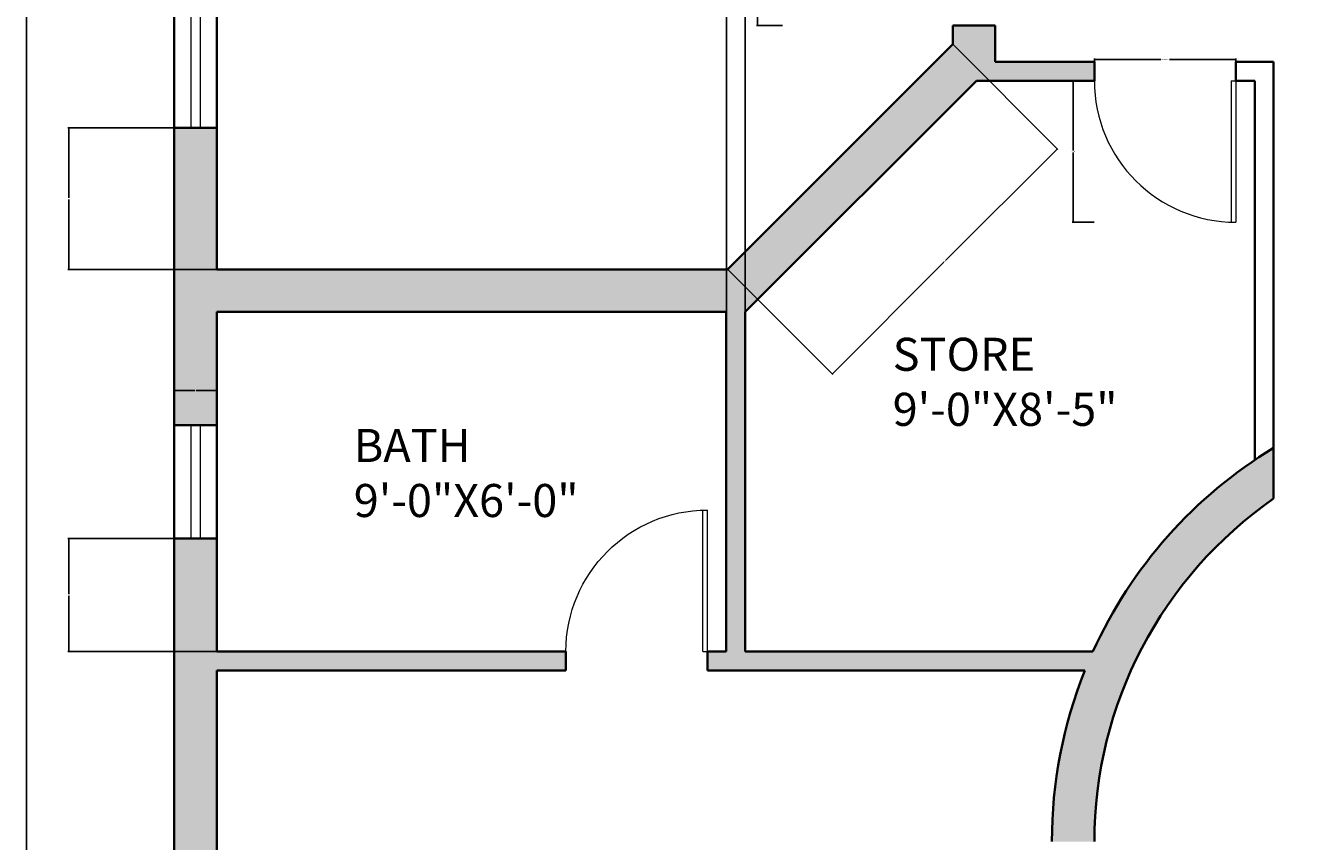
# Model space of a CAD drawing. Units: inches. Extents: x 1919 to 2461, y 2470 to 3159.
# Tile 2 of 6: x 1919 to 2188, y 2630 to 2803. Entities that reach past the tile are written whole.
import ezdxf

# ---------------------------------------------------------------- set-up
doc = ezdxf.new("R2010")
doc.units = ezdxf.units.IN
for name, color, linetype, lineweight in [('A-ANNO-DIMS', 2, 'Continuous', 18), ('A-AREA-IDEN', 7, 'Continuous', 18), ('A-DOOR', 3, 'Continuous', 18), ('A-GLAZ', 4, 'Continuous', 18), ('A-WALL', 7, 'Continuous', 35), ('A-WALL-PATT', 252, 'Continuous', 13)]:
    doc.layers.add(name, color=color, linetype=linetype, lineweight=lineweight)
doc.styles.get("Standard").update_dxf_attribs({"font": 'arial.ttf'})
doc.dimstyles.get("Standard").update_dxf_attribs({"dimtxt": 0.18, "dimasz": 0.18, "dimexe": 0.18, "dimexo": 0.0625, "dimgap": 0.09, "dimtad": 0, "dimtih": 1, "dimtoh": 1, "dimdec": 4, "dimzin": 0, "dimdsep": 46, "dimtxsty": 'Standard', "dimcen": 0.09, "dimadec": 0, "dimazin": 0, "dimtfac": 1, "dimtdec": 4, "dimtofl": 0, "dimtmove": 0, "dimatfit": 3, "dimfxl": 1, "dimtolj": 1, "dimtzin": 0, "dimarcsym": 0})

# ---------------------------------------------------------------- blocks, each defined once
blk = doc.blocks.new('DOOR-SGL-30IN')
for p, q in [((0, 0), (0, 30)), ((1, 0), (1, 29.98)), ((1, 0), (0, 0))]:
    blk.add_line(p, q)
blk.add_arc((0, 0), 30, 0, 90)
blk = doc.blocks.new('WIN-GLAZ-120IN')
for p, q in [((120, 0), (0, 0)), ((120, -2), (0, -2))]:
    blk.add_line(p, q)
blk = doc.blocks.new('WIN-GLAZ-24IN')
for p, q in [((-2, 24), (-2, 0)), ((0, 24), (0, 0))]:
    blk.add_line(p, q)
blk = doc.blocks.new('*D14')
at = {"layer": 'A-ANNO-DIMS', "color": 0, "lineweight": -2, "transparency": 16777216}
for p, q in [((2079.25, 2839.4), (2073.74, 2839.4)), ((2073.92, 2839.22), (2073.92, 2821.58)), ((2073.92, 2803.58), (2073.92, 2821.22)), ((2079.25, 2803.4), (2073.74, 2803.4))]:
    blk.add_line(p, q, dxfattribs=at)
at = {"layer": 'A-ANNO-DIMS', "color": 0, "transparency": 16777216}
for points in [[(2073.89, 2839.22), (2073.95, 2839.22), (2073.92, 2839.4)], [(2073.89, 2803.58), (2073.95, 2803.58), (2073.92, 2803.4)]]:
    blk.add_solid(points, dxfattribs=at)
at = {"layer": 'Defpoints', "color": 0, "transparency": 16777216}
for p in [(2073.92, 2839.4), (2079.32, 2839.4), (2079.32, 2803.4)]:
    blk.add_point(p, dxfattribs=at)
at = {"layer": 'A-ANNO-DIMS', "color": 0, "transparency": 16777216, "insert": (2073.92, 2821.4), "char_height": 0.18, "attachment_point": 5}
blk.add_mtext('\\A1;36 TYP.', dxfattribs=at)
blk = doc.blocks.new('*D15')
at = {"layer": 'A-ANNO-DIMS', "color": 0, "lineweight": -2, "transparency": 16777216}
for p, q in [((2145.32, 2791.73), (2145.32, 2796.35)), ((2145.5, 2796.17), (2159.38, 2796.17)), ((2175.14, 2796.17), (2161.25, 2796.17)), ((2175.32, 2791.73), (2175.32, 2796.35))]:
    blk.add_line(p, q, dxfattribs=at)
at = {"layer": 'A-ANNO-DIMS', "color": 0, "transparency": 16777216}
for points in [[(2145.5, 2796.2), (2145.5, 2796.14), (2145.32, 2796.17)], [(2175.14, 2796.2), (2175.14, 2796.14), (2175.32, 2796.17)]]:
    blk.add_solid(points, dxfattribs=at)
at = {"layer": 'Defpoints', "color": 0, "transparency": 16777216}
for p in [(2145.32, 2796.17), (2145.32, 2791.67), (2175.32, 2791.67)]:
    blk.add_point(p, dxfattribs=at)
at = {"layer": 'A-ANNO-DIMS', "color": 0, "transparency": 16777216, "insert": (2160.32, 2796.17), "char_height": 0.18, "attachment_point": 5}
blk.add_mtext('\\A1;DOOR 30 TYP.', dxfattribs=at)
blk = doc.blocks.new('*D16')
at = {"layer": 'A-ANNO-DIMS', "color": 0, "lineweight": -2, "transparency": 16777216}
for p, q in [((2145.25, 2791.67), (2140.64, 2791.67)), ((2140.82, 2791.49), (2140.82, 2776.85)), ((2140.82, 2761.85), (2140.82, 2776.49)), ((2145.25, 2761.67), (2140.64, 2761.67))]:
    blk.add_line(p, q, dxfattribs=at)
at = {"layer": 'A-ANNO-DIMS', "color": 0, "transparency": 16777216}
for points in [[(2140.79, 2791.49), (2140.85, 2791.49), (2140.82, 2791.67)], [(2140.79, 2761.85), (2140.85, 2761.85), (2140.82, 2761.67)]]:
    blk.add_solid(points, dxfattribs=at)
at = {"layer": 'Defpoints', "color": 0, "transparency": 16777216}
for p in [(2145.32, 2791.67), (2140.82, 2761.67), (2145.32, 2761.67)]:
    blk.add_point(p, dxfattribs=at)
at = {"layer": 'A-ANNO-DIMS', "color": 0, "transparency": 16777216, "insert": (2140.82, 2776.67), "char_height": 0.18, "attachment_point": 5}
blk.add_mtext('\\A1;30 TYP.', dxfattribs=at)
blk = doc.blocks.new('*D24')
at = {"layer": 'A-ANNO-DIMS', "color": 0, "lineweight": -2, "transparency": 16777216}
for p, q in [((2004.25, 3127.67), (1918.78, 3127.67)), ((1918.96, 3127.49), (1918.96, 2814.85)), ((1918.96, 2501.85), (1918.96, 2814.49)), ((1950.25, 2501.67), (1918.78, 2501.67))]:
    blk.add_line(p, q, dxfattribs=at)
at = {"layer": 'A-ANNO-DIMS', "color": 0, "transparency": 16777216}
for points in [[(1918.93, 3127.49), (1918.99, 3127.49), (1918.96, 3127.67)], [(1918.93, 2501.85), (1918.99, 2501.85), (1918.96, 2501.67)]]:
    blk.add_solid(points, dxfattribs=at)
at = {"layer": 'Defpoints', "color": 0, "transparency": 16777216}
for p in [(1918.96, 3127.67), (2004.32, 3127.67), (1950.32, 2501.67)]:
    blk.add_point(p, dxfattribs=at)
at = {"layer": 'A-ANNO-DIMS', "color": 0, "transparency": 16777216, "insert": (1918.96, 2814.67), "char_height": 0.18, "attachment_point": 5}
blk.add_mtext('\\A1;626', dxfattribs=at)
blk = doc.blocks.new('*D30')
at = {"layer": 'A-ANNO-DIMS', "color": 0, "lineweight": -2, "transparency": 16777216}
for p, q in [((1959.25, 2781.67), (1927.78, 2781.67)), ((1927.96, 2781.49), (1927.96, 2766.85)), ((1927.96, 2751.85), (1927.96, 2766.49)), ((1959.25, 2751.67), (1927.78, 2751.67))]:
    blk.add_line(p, q, dxfattribs=at)
at = {"layer": 'A-ANNO-DIMS', "color": 0, "transparency": 16777216}
for points in [[(1927.93, 2781.49), (1927.99, 2781.49), (1927.96, 2781.67)], [(1927.93, 2751.85), (1927.99, 2751.85), (1927.96, 2751.67)]]:
    blk.add_solid(points, dxfattribs=at)
at = {"layer": 'Defpoints', "color": 0, "transparency": 16777216}
for p in [(1927.96, 2781.67), (1959.32, 2781.67), (1959.32, 2751.67)]:
    blk.add_point(p, dxfattribs=at)
at = {"layer": 'A-ANNO-DIMS', "color": 0, "transparency": 16777216, "insert": (1927.96, 2766.67), "char_height": 0.18, "attachment_point": 5}
blk.add_mtext('\\A1;30', dxfattribs=at)
blk = doc.blocks.new('*D31')
at = {"layer": 'A-ANNO-DIMS', "color": 0, "lineweight": -2, "transparency": 16777216}
for p, q in [((1959.25, 2694.67), (1927.78, 2694.67)), ((1927.96, 2694.49), (1927.96, 2682.85)), ((1927.96, 2670.85), (1927.96, 2682.49)), ((1959.25, 2670.67), (1927.78, 2670.67))]:
    blk.add_line(p, q, dxfattribs=at)
at = {"layer": 'A-ANNO-DIMS', "color": 0, "transparency": 16777216}
for points in [[(1927.93, 2694.49), (1927.99, 2694.49), (1927.96, 2694.67)], [(1927.93, 2670.85), (1927.99, 2670.85), (1927.96, 2670.67)]]:
    blk.add_solid(points, dxfattribs=at)
at = {"layer": 'Defpoints', "color": 0, "transparency": 16777216}
for p in [(1927.96, 2694.67), (1959.32, 2694.67), (1959.32, 2670.67)]:
    blk.add_point(p, dxfattribs=at)
at = {"layer": 'A-ANNO-DIMS', "color": 0, "transparency": 16777216, "insert": (1927.96, 2682.67), "char_height": 0.18, "attachment_point": 5}
blk.add_mtext('\\A1;24', dxfattribs=at)
blk = doc.blocks.new('*D39')
at = {"layer": 'A-ANNO-DIMS', "color": 0, "lineweight": -2, "transparency": 16777216}
for p, q in [((2067.32, 2670.73), (2067.32, 3159.21)), ((2067.5, 3159.03), (2069.16, 3159.03)), ((2071.14, 3159.03), (2069.47, 3159.03)), ((2071.32, 2670.73), (2071.32, 3159.21))]:
    blk.add_line(p, q, dxfattribs=at)
at = {"layer": 'A-ANNO-DIMS', "color": 0, "transparency": 16777216}
for points in [[(2067.5, 3159.06), (2067.5, 3159), (2067.32, 3159.03)], [(2071.14, 3159.06), (2071.14, 3159), (2071.32, 3159.03)]]:
    blk.add_solid(points, dxfattribs=at)
at = {"layer": 'Defpoints', "color": 0, "transparency": 16777216}
for p in [(2071.32, 3159.03), (2067.32, 2670.67), (2071.32, 2670.67)]:
    blk.add_point(p, dxfattribs=at)
at = {"layer": 'A-ANNO-DIMS', "color": 0, "transparency": 16777216, "insert": (2069.32, 3159.03), "char_height": 0.18, "attachment_point": 5}
blk.add_mtext('\\A1;4', dxfattribs=at)
blk = doc.blocks.new('*D40')
at = {"layer": 'A-ANNO-DIMS', "color": 0, "lineweight": -2, "transparency": 16777216}
for p, q in [((1950.32, 2694.73), (1950.32, 2726.21)), ((1950.5, 2726.03), (1954.67, 2726.03)), ((1959.14, 2726.03), (1954.96, 2726.03)), ((1959.32, 2694.73), (1959.32, 2726.21))]:
    blk.add_line(p, q, dxfattribs=at)
at = {"layer": 'A-ANNO-DIMS', "color": 0, "transparency": 16777216}
for points in [[(1950.5, 2726.06), (1950.5, 2726), (1950.32, 2726.03)], [(1959.14, 2726.06), (1959.14, 2726), (1959.32, 2726.03)]]:
    blk.add_solid(points, dxfattribs=at)
at = {"layer": 'Defpoints', "color": 0, "transparency": 16777216}
for p in [(1959.32, 2726.03), (1950.32, 2694.67), (1959.32, 2694.67)]:
    blk.add_point(p, dxfattribs=at)
at = {"layer": 'A-ANNO-DIMS', "color": 0, "transparency": 16777216, "insert": (1954.82, 2726.03), "char_height": 0.18, "attachment_point": 5}
blk.add_mtext('\\A1;9', dxfattribs=at)
blk = doc.blocks.new('*D44')
at = {"layer": 'A-ANNO-DIMS', "color": 0, "lineweight": -2, "transparency": 16777216}
for p, q in [((2115.36, 2799.36), (2137.61, 2777.1)), ((2137.36, 2777.1), (2113.8, 2753.55)), ((2089.89, 2729.63), (2113.44, 2753.18)), ((2067.63, 2751.63), (2089.89, 2729.37))]:
    blk.add_line(p, q, dxfattribs=at)
at = {"layer": 'A-ANNO-DIMS', "color": 0, "transparency": 16777216}
for points in [[(2137.34, 2777.12), (2137.38, 2777.08), (2137.49, 2777.23)], [(2089.86, 2729.65), (2089.91, 2729.61), (2089.76, 2729.5)]]:
    blk.add_solid(points, dxfattribs=at)
at = {"layer": 'Defpoints', "color": 0, "transparency": 16777216}
for p in [(2115.32, 2799.4), (2067.59, 2751.67), (2089.76, 2729.5)]:
    blk.add_point(p, dxfattribs=at)
at = {"layer": 'A-ANNO-DIMS', "color": 0, "transparency": 16777216, "insert": (2113.62, 2753.36), "char_height": 0.18, "attachment_point": 5}
blk.add_mtext('\\A1;67.5', dxfattribs=at)

msp = doc.modelspace()

# ---------------------------------------------------------------- hatches: boundary and pattern name
at = {"layer": 'A-WALL-PATT'}
h = msp.add_hatch(color=256, dxfattribs=at)
h.dxf.hatch_style = 1
h.paths.add_polyline_path([(1959.315, 2931.672), (2066.315, 2931.672), (2066.315, 2940.672), (2062.315, 2940.672), (2062.315, 3005.672), (2066.315, 3005.672), (2066.315, 3009.672), (2062.315, 3009.672), (2062.315, 3118.672), (2062.315, 3127.672), (2004.315, 3127.672), (2004.315, 3072.672), (1950.315, 3072.672), (1950.315, 3059.672), (1959.315, 3059.672), (1959.315, 3063.672), (2017.315, 3063.672), (2017.315, 3067.672), (2013.315, 3067.672), (2013.315, 3118.672), (2058.315, 3118.672), (2058.315, 3067.672), (2047.315, 3067.672), (2047.315, 3063.672), (2058.315, 3063.672), (2058.315, 2940.672), (1959.315, 2940.672), (1959.315, 2952.172), (1950.315, 2952.172), (1950.315, 2901.672), (1959.315, 2901.672)])
h.paths.add_polyline_path([(2120.315, 2791.672), (2145.315, 2791.672), (2145.315, 2795.672), (2124.315, 2795.672), (2124.315, 2803.3999), (2115.315, 2803.3999), (2115.315, 2799.3999), (2067.5871, 2751.672), (1959.315, 2751.672), (1959.315, 2781.672), (1950.315, 2781.672), (1950.315, 2718.672), (1959.315, 2718.672), (1959.315, 2742.672), (2067.315, 2742.672), (2067.315, 2670.672), (2063.315, 2670.672), (2063.315, 2666.672), (2143.3108, 2666.672, 0.09553844), (2136.315, 2630.3938), (2145.315, 2630.3938, -0.2455558), (2183.315, 2703.1037), (2183.315, 2713.8315, 0.15123975), (2145.0175, 2670.672), (2071.315, 2670.672), (2071.315, 2742.672)])
h.paths.add_polyline_path([(2124.315, 2931.672), (2232.315, 2931.672), (2232.315, 2940.672), (2228.315, 2940.672), (2228.315, 2964.672), (2219.315, 2964.672), (2219.315, 2940.672), (2138.315, 2940.672), (2138.315, 3005.672), (2185.315, 3005.672), (2185.315, 3009.672), (2138.315, 3009.672), (2138.315, 3118.672), (2138.315, 3127.672), (2086.315, 3127.672), (2086.315, 3118.672), (2134.315, 3118.672), (2134.315, 3009.672), (2096.315, 3009.672), (2096.315, 3005.672), (2134.315, 3005.672), (2134.315, 2940.672), (2096.315, 2940.672), (2096.315, 2931.672), (2115.315, 2931.672), (2115.315, 2839.3999), (2124.315, 2839.3999)])
h.paths.add_polyline_path([(2429.315, 3127.672), (2384.315, 3127.672), (2384.315, 3118.672), (2420.315, 3118.672), (2420.315, 2940.672), (2268.315, 2940.672), (2268.315, 2931.672), (2420.315, 2931.672), (2420.315, 2727.672), (2364.3064, 2727.672), (2317.4188, 2680.7844, 0.0404216), (2308.2227, 2693.5694), (2301.7735, 2687.2567, -0.63673951), (2233.8773, 2541.8315), (2145.315, 2541.8315), (2145.315, 2594.3938), (2136.315, 2594.3938), (2136.315, 2510.672), (2107.815, 2510.672), (2107.815, 2501.672), (2145.315, 2501.672), (2145.315, 2532.8315), (2233.8773, 2532.8315, 0.55190633), (2321.8781, 2672.5158), (2368.0343, 2718.672), (2429.315, 2718.672)])
h.paths.add_polyline_path([(2228.315, 3118.672), (2264.315, 3118.672), (2264.315, 3127.672), (2162.315, 3127.672), (2162.315, 3118.672), (2219.315, 3118.672), (2219.315, 3009.672), (2215.315, 3009.672), (2215.315, 3005.672), (2219.315, 3005.672), (2219.315, 2994.672), (2228.315, 2994.672)], flags=0)
h.paths.add_polyline_path([(1959.315, 2666.672), (2033.315, 2666.672), (2033.315, 2670.672), (1959.315, 2670.672), (1959.315, 2694.672), (1950.315, 2694.672), (1950.315, 2501.672), (1987.815, 2501.672), (1987.815, 2510.672), (1959.315, 2510.672)])

# ---------------------------------------------------------------- linework, layer by layer
at = {"layer": 'A-WALL'}
for p, q in [((1950.315, 3023.672), (1950.315, 2501.672)), ((1959.315, 2751.672), (1959.315, 2931.672)), ((2115.315, 2799.3999), (2115.315, 2803.3999)), ((2115.315, 2803.3999), (2124.315, 2803.3999)), ((2124.315, 2795.672), (2124.315, 2803.3999)), ((2067.5871, 2751.672), (2115.315, 2799.3999)), ((2124.315, 2795.672), (2145.315, 2795.672)), ((2145.315, 2791.672), (2145.315, 2795.672)), ((2175.315, 2791.672), (2175.315, 2795.672)), ((2175.315, 2795.672), (2183.315, 2795.672)), ((2183.315, 2703.1037), (2183.315, 2795.672)), ((2071.315, 2742.672), (2120.315, 2791.672)), ((2120.315, 2791.672), (2145.315, 2791.672)), ((2175.315, 2791.672), (2179.315, 2791.672)), ((2179.315, 2711.2724), (2179.315, 2791.672)), ((1959.315, 2781.672), (1950.315, 2781.672)), ((1959.315, 2751.672), (2067.5871, 2751.672)), ((1959.315, 2742.672), (2067.315, 2742.672)), ((1959.315, 2670.672), (1959.315, 2742.672)), ((2067.315, 2670.672), (2067.315, 2742.672)), ((2071.315, 2670.672), (2071.315, 2742.672)), ((1959.315, 2718.672), (1950.315, 2718.672)), ((1959.315, 2694.672), (1950.315, 2694.672)), ((1959.315, 2670.672), (2033.315, 2670.672)), ((2033.315, 2666.672), (2033.315, 2670.672)), ((2063.315, 2666.672), (2063.315, 2670.672)), ((2063.315, 2670.672), (2067.315, 2670.672)), ((2071.315, 2670.672), (2145.0175, 2670.672)), ((1959.315, 2666.672), (1959.315, 2510.672)), ((1959.315, 2666.672), (2033.315, 2666.672)), ((2063.315, 2666.672), (2143.3108, 2666.672))]:
    msp.add_line(p, q, dxfattribs=at)
for radius, start, end in [(97.5623, 121.215371, 155.616261), (88.5623, 124.814645, 180), (97.5623, 158.170458, 180)]:
    msp.add_arc((2233.8773, 2630.3938), radius, start, end, dxfattribs=at)

# ---------------------------------------------------------------- block references
at = {"layer": 'A-DOOR', "rotation": 180}
msp.add_blockref('DOOR-SGL-30IN', (2175.315, 2791.672), dxfattribs=at)
at = {"layer": 'A-DOOR', "extrusion": (0, 0, -1), "zscale": -1}
msp.add_blockref('DOOR-SGL-30IN', (-2063.315, 2670.672), dxfattribs=at)
at = {"layer": 'A-GLAZ', "rotation": 90}
msp.add_blockref('WIN-GLAZ-120IN', (1953.815, 2781.672), dxfattribs=at)
at = {"layer": 'A-GLAZ'}
msp.add_blockref('WIN-GLAZ-24IN', (1955.815, 2694.672), dxfattribs=at)

# ---------------------------------------------------------------- texts
at = {"layer": 'A-AREA-IDEN', "char_height": 7, "attachment_point": 1}
for s, insert in [('STORE\\P9\'-0"X8\'-5"', (2102.5773, 2737.189)), ('BATH\\P9\'-0"X6\'-0"', (1988.3513, 2717.8622))]:
    msp.add_mtext_dynamic_manual_height_columns(s, width=121.344683, gutter_width=12.5, heights=[0], dxfattribs=dict(at, insert=insert))

# ---------------------------------------------------------------- dimensions: what is measured, and where the dimension line sits
at = {"layer": 'A-ANNO-DIMS'}
for base, p1, p2, picture, middle in [((2071.315, 3159.027), (2067.315, 2670.672), (2071.315, 2670.672), '*D39', (2069.315, 3159.027)), ((1959.315, 2726.027), (1950.315, 2694.672), (1959.315, 2694.672), '*D40', (1954.815, 2726.027))]:
    dim = msp.add_linear_dim(base=base, p1=p1, p2=p2, dimstyle='Standard', override={"dimdec": 0, "dimlfac": 1, "dimrnd": 0, "dimzin": 0, "dimdsep": 46, "dimlunit": 2}, dxfattribs=at)
    dim.commit()
    dim.dimension.update_dxf_attribs({"geometry": picture, "text_midpoint": middle})
for base, p1, p2, angle, override, picture, middle in [((1918.96, 3127.672), (1950.315, 2501.672), (2004.315, 3127.672), 90, {"dimdec": 0, "dimlfac": 1, "dimrnd": 0, "dimzin": 0, "dimdsep": 46, "dimlunit": 2}, '*D24', (1918.96, 2814.672)), ((2089.7584, 2729.5007), (2115.315, 2799.3999), (2067.5871, 2751.672), 225, {"dimdec": 1, "dimlfac": 1, "dimrnd": 0, "dimzin": 0, "dimdsep": 46, "dimlunit": 2}, '*D44', (2113.6224, 2753.3646)), ((1927.96, 2781.672), (1959.315, 2751.672), (1959.315, 2781.672), 90, {"dimdec": 0, "dimlfac": 1, "dimrnd": 0, "dimzin": 0, "dimdsep": 46, "dimlunit": 2}, '*D30', (1927.96, 2766.672)), ((1927.96, 2694.672), (1959.315, 2670.672), (1959.315, 2694.672), 90, {"dimdec": 0, "dimlfac": 1, "dimrnd": 0, "dimzin": 0, "dimdsep": 46, "dimlunit": 2}, '*D31', (1927.96, 2682.672))]:
    dim = msp.add_linear_dim(base=base, p1=p1, p2=p2, angle=angle, dimstyle='Standard', override=override, dxfattribs=at)
    dim.commit()
    dim.dimension.update_dxf_attribs({"geometry": picture, "text_midpoint": middle})
for base, p1, p2, angle, text, picture, middle in [((2073.915, 2839.3999), (2079.315, 2803.3999), (2079.315, 2839.3999), 90, '<> TYP.', '*D14', (2073.915, 2821.3999)), ((2145.315, 2796.172), (2175.315, 2791.672), (2145.315, 2791.672), 180, 'DOOR <> TYP.', '*D15', (2160.315, 2796.172)), ((2140.815, 2761.672), (2145.315, 2791.672), (2145.315, 2761.672), 270, '<> TYP.', '*D16', (2140.815, 2776.672))]:
    dim = msp.add_linear_dim(base=base, p1=p1, p2=p2, angle=angle, text=text, dimstyle='Standard', override={"dimdec": 0, "dimlfac": 1, "dimrnd": 0, "dimzin": 0, "dimdsep": 46, "dimlunit": 2}, dxfattribs=at)
    dim.commit()
    dim.dimension.update_dxf_attribs({"geometry": picture, "text_midpoint": middle})

doc.saveas('drawing.dxf')
